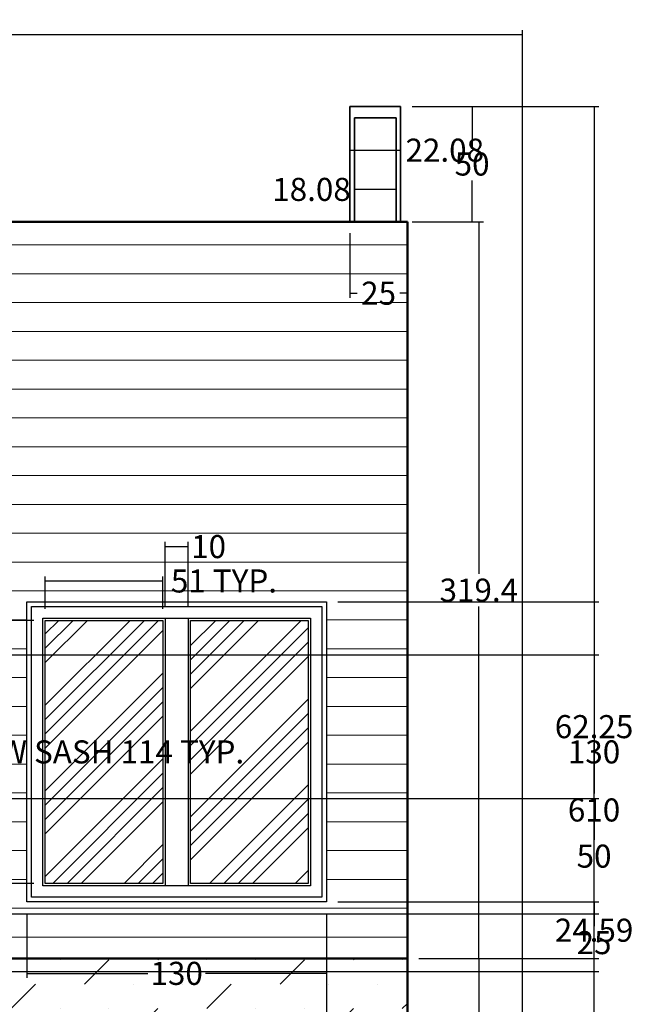
# Model space of a CAD drawing. Units: millimetres. Extents: x 301 to 1039, y -12 to 673.
# Tile 6 of 6: x 736 to 1002, y 246 to 673. Entities that reach past the tile are written whole.
import ezdxf

# ---------------------------------------------------------------- set-up
doc = ezdxf.new("R2010")
doc.units = ezdxf.units.MM
doc.header["$MEASUREMENT"] = 0
for name, color, linetype, lineweight in [('A-ANNO-DIMS', 2, 'Continuous', 18), ('A-GLAZ', 4, 'Continuous', 25), ('A-GLAZ-PATT', 8, 'Continuous', 13), ('A-ROOF', 1, 'Continuous', 35), ('A-WALL', 7, 'Continuous', 50), ('A-WALL-PATT', 9, 'Continuous', 13)]:
    doc.layers.add(name, color=color, linetype=linetype, lineweight=lineweight)
doc.styles.get("Standard").update_dxf_attribs({"font": 'arial.ttf'})
doc.dimstyles.get("Standard").update_dxf_attribs({"dimtxt": 10, "dimasz": 0.18, "dimexe": 2, "dimexo": 5, "dimgap": 2, "dimtad": 0, "dimtih": 1, "dimtoh": 1, "dimdec": 0, "dimzin": 0, "dimdsep": 46, "dimtxsty": 'Standard', "dimcen": 0.09, "dimadec": 0, "dimazin": 0, "dimtfac": 1, "dimtdec": 0, "dimtofl": 0, "dimtmove": 0, "dimatfit": 3, "dimfxl": 1, "dimtolj": 1, "dimtzin": 0, "dimarcsym": 0})

# ---------------------------------------------------------------- blocks, each defined once
blk = doc.blocks.new('WIN-SASH-SLIDING')
blk.add_line((51, 114), (51, 0))
blk.add_lwpolyline([(51, 0), (0, 0), (0, 114), (51, 114)])
blk = doc.blocks.new('*D16')
at = {"layer": 'A-ANNO-DIMS', "color": 0, "lineweight": -2, "transparency": 16777216}
for p, q in [((741.69, 412.26), (727.59, 412.26)), ((729.59, 412.08), (729.59, 362.44)), ((729.59, 298.44), (729.59, 348.09)), ((741.69, 298.26), (727.59, 298.26))]:
    blk.add_line(p, q, dxfattribs=at)
at = {"layer": 'A-ANNO-DIMS', "color": 0, "transparency": 16777216}
for points in [[(729.56, 412.08), (729.62, 412.08), (729.59, 412.26)], [(729.56, 298.44), (729.62, 298.44), (729.59, 298.26)]]:
    blk.add_solid(points, dxfattribs=at)
at = {"layer": 'Defpoints', "color": 0, "transparency": 16777216}
for p in [(729.59, 412.26), (746.69, 412.26), (746.69, 298.26)]:
    blk.add_point(p, dxfattribs=at)
at = {"layer": 'A-ANNO-DIMS', "color": 0, "transparency": 16777216, "insert": (729.59, 355.26), "char_height": 10, "attachment_point": 5}
blk.add_mtext('\\A1;SLIDING WINDOW SASH 114 TYP.', dxfattribs=at)
blk = doc.blocks.new('*D17')
at = {"layer": 'A-ANNO-DIMS', "color": 0, "lineweight": -2, "transparency": 16777216}
for p, q in [((746.69, 417.26), (746.69, 431.36)), ((797.69, 417.26), (797.69, 431.36)), ((746.87, 429.36), (797.51, 429.36)), ((797.69, 429.36), (797.87, 429.36))]:
    blk.add_line(p, q, dxfattribs=at)
at = {"layer": 'A-ANNO-DIMS', "color": 0, "transparency": 16777216}
for points in [[(746.87, 429.39), (746.87, 429.33), (746.69, 429.36)], [(797.51, 429.39), (797.51, 429.33), (797.69, 429.36)]]:
    blk.add_solid(points, dxfattribs=at)
at = {"layer": 'Defpoints', "color": 0, "transparency": 16777216}
for p in [(797.69, 429.36), (746.69, 412.26), (797.69, 412.26)]:
    blk.add_point(p, dxfattribs=at)
at = {"layer": 'A-ANNO-DIMS', "color": 0, "transparency": 16777216, "insert": (824.21, 429.36), "char_height": 10, "attachment_point": 5}
blk.add_mtext('\\A1;51 TYP.', dxfattribs=at)
blk = doc.blocks.new('*D20')
at = {"layer": 'A-ANNO-DIMS', "color": 0, "lineweight": -2, "transparency": 16777216}
for p, q in [((343.79, 30.09), (343.79, 668.09)), ((343.97, 666.09), (635.73, 666.09)), ((953.61, 666.09), (661.85, 666.09)), ((953.79, 30.09), (953.79, 668.09))]:
    blk.add_line(p, q, dxfattribs=at)
at = {"layer": 'A-ANNO-DIMS', "color": 0, "transparency": 16777216}
for points in [[(343.97, 666.12), (343.97, 666.06), (343.79, 666.09)], [(953.61, 666.12), (953.61, 666.06), (953.79, 666.09)]]:
    blk.add_solid(points, dxfattribs=at)
at = {"layer": 'Defpoints', "color": 0, "transparency": 16777216}
for p in [(953.79, 666.09), (343.79, 25.09), (953.79, 25.09)]:
    blk.add_point(p, dxfattribs=at)
at = {"layer": 'A-ANNO-DIMS', "color": 0, "transparency": 16777216, "insert": (648.79, 666.09), "char_height": 10, "attachment_point": 5}
blk.add_mtext('\\A1;610', dxfattribs=at)
blk = doc.blocks.new('*D21')
at = {"layer": 'A-ANNO-DIMS', "color": 0, "lineweight": -2, "transparency": 16777216}
for p, q in [((905.87, 635.09), (986.79, 635.09)), ((984.79, 634.91), (984.79, 337.19)), ((984.79, 25.27), (984.79, 322.98)), ((958.79, 25.09), (986.79, 25.09))]:
    blk.add_line(p, q, dxfattribs=at)
at = {"layer": 'A-ANNO-DIMS', "color": 0, "transparency": 16777216}
for points in [[(984.76, 634.91), (984.82, 634.91), (984.79, 635.09)], [(984.76, 25.27), (984.82, 25.27), (984.79, 25.09)]]:
    blk.add_solid(points, dxfattribs=at)
at = {"layer": 'Defpoints', "color": 0, "transparency": 16777216}
for p in [(900.87, 635.09), (984.79, 635.09), (953.79, 25.09)]:
    blk.add_point(p, dxfattribs=at)
at = {"layer": 'A-ANNO-DIMS', "color": 0, "transparency": 16777216, "insert": (984.79, 330.09), "char_height": 10, "attachment_point": 5}
blk.add_mtext('\\A1;610', dxfattribs=at)
blk = doc.blocks.new('*D38')
at = {"layer": 'A-ANNO-DIMS', "color": 0, "lineweight": -2, "transparency": 16777216}
for p, q in [((908.79, 265.67), (936.79, 265.67)), ((934.79, 265.49), (934.79, 157.49)), ((934.79, 35.27), (934.79, 143.27)), ((908.79, 35.09), (936.79, 35.09))]:
    blk.add_line(p, q, dxfattribs=at)
at = {"layer": 'A-ANNO-DIMS', "color": 0, "transparency": 16777216}
for points in [[(934.76, 265.49), (934.82, 265.49), (934.79, 265.67)], [(934.76, 35.27), (934.82, 35.27), (934.79, 35.09)]]:
    blk.add_solid(points, dxfattribs=at)
at = {"layer": 'Defpoints', "color": 0, "transparency": 16777216}
for p in [(903.79, 265.67), (903.79, 35.09), (934.79, 35.09)]:
    blk.add_point(p, dxfattribs=at)
at = {"layer": 'A-ANNO-DIMS', "color": 0, "transparency": 16777216, "insert": (934.79, 150.38), "char_height": 10, "attachment_point": 5}
blk.add_mtext('\\A1;230.6', dxfattribs=at)
blk = doc.blocks.new('*D39')
at = {"layer": 'A-ANNO-DIMS', "color": 0, "lineweight": -2, "transparency": 16777216}
for p, q in [((908.79, 585.09), (936.79, 585.09)), ((934.79, 584.91), (934.79, 432.49)), ((934.79, 265.85), (934.79, 418.27)), ((908.79, 265.67), (936.79, 265.67))]:
    blk.add_line(p, q, dxfattribs=at)
at = {"layer": 'A-ANNO-DIMS', "color": 0, "transparency": 16777216}
for points in [[(934.76, 584.91), (934.82, 584.91), (934.79, 585.09)], [(934.76, 265.85), (934.82, 265.85), (934.79, 265.67)]]:
    blk.add_solid(points, dxfattribs=at)
at = {"layer": 'Defpoints', "color": 0, "transparency": 16777216}
for p in [(903.79, 585.09), (903.79, 265.67), (934.79, 265.67)]:
    blk.add_point(p, dxfattribs=at)
at = {"layer": 'A-ANNO-DIMS', "color": 0, "transparency": 16777216, "insert": (934.79, 425.38), "char_height": 10, "attachment_point": 5}
blk.add_mtext('\\A1;319.4', dxfattribs=at)
blk = doc.blocks.new('*D46')
at = {"layer": 'A-ANNO-DIMS', "color": 0, "lineweight": -2, "transparency": 16777216}
for p, q in [((878.79, 590.09), (878.79, 618.09)), ((878.97, 616.09), (900.69, 616.09)), ((900.87, 590.09), (900.87, 618.09)), ((900.87, 616.09), (901.05, 616.09))]:
    blk.add_line(p, q, dxfattribs=at)
at = {"layer": 'A-ANNO-DIMS', "color": 0, "transparency": 16777216}
for points in [[(878.97, 616.12), (878.97, 616.06), (878.79, 616.09)], [(900.69, 616.12), (900.69, 616.06), (900.87, 616.09)]]:
    blk.add_solid(points, dxfattribs=at)
at = {"layer": 'Defpoints', "color": 0, "transparency": 16777216}
for p in [(900.87, 616.09), (878.79, 585.09), (900.87, 585.09)]:
    blk.add_point(p, dxfattribs=at)
at = {"layer": 'A-ANNO-DIMS', "color": 0, "transparency": 16777216, "insert": (920.02, 616.09), "char_height": 10, "attachment_point": 5}
blk.add_mtext('\\A1;22.08', dxfattribs=at)
blk = doc.blocks.new('*D47')
at = {"layer": 'A-ANNO-DIMS', "color": 0, "lineweight": -2, "transparency": 16777216}
for p, q in [((880.79, 625.09), (880.79, 597.09)), ((898.87, 625.09), (898.87, 597.09)), ((880.79, 599.09), (880.61, 599.09)), ((898.69, 599.09), (880.97, 599.09))]:
    blk.add_line(p, q, dxfattribs=at)
at = {"layer": 'A-ANNO-DIMS', "color": 0, "transparency": 16777216}
for points in [[(880.97, 599.12), (880.97, 599.06), (880.79, 599.09)], [(898.69, 599.12), (898.69, 599.06), (898.87, 599.09)]]:
    blk.add_solid(points, dxfattribs=at)
at = {"layer": 'Defpoints', "color": 0, "transparency": 16777216}
for p in [(880.79, 630.09), (898.87, 630.09), (880.79, 599.09)]:
    blk.add_point(p, dxfattribs=at)
at = {"layer": 'A-ANNO-DIMS', "color": 0, "transparency": 16777216, "insert": (862.2, 599.09), "char_height": 10, "attachment_point": 5}
blk.add_mtext('\\A1;18.08', dxfattribs=at)
blk = doc.blocks.new('*D48')
at = {"layer": 'A-ANNO-DIMS', "color": 0, "lineweight": -2, "transparency": 16777216}
for p, q in [((878.79, 580.09), (878.79, 552.09)), ((903.79, 580.09), (903.79, 552.09)), ((878.97, 554.09), (882, 554.09)), ((903.61, 554.09), (900.57, 554.09))]:
    blk.add_line(p, q, dxfattribs=at)
at = {"layer": 'A-ANNO-DIMS', "color": 0, "transparency": 16777216}
for points in [[(878.97, 554.12), (878.97, 554.06), (878.79, 554.09)], [(903.61, 554.12), (903.61, 554.06), (903.79, 554.09)]]:
    blk.add_solid(points, dxfattribs=at)
at = {"layer": 'Defpoints', "color": 0, "transparency": 16777216}
for p in [(878.79, 585.09), (903.79, 585.09), (878.79, 554.09)]:
    blk.add_point(p, dxfattribs=at)
at = {"layer": 'A-ANNO-DIMS', "color": 0, "transparency": 16777216, "insert": (891.29, 554.09), "char_height": 10, "attachment_point": 5}
blk.add_mtext('\\A1;25', dxfattribs=at)
blk = doc.blocks.new('*D49')
at = {"layer": 'A-ANNO-DIMS', "color": 0, "lineweight": -2, "transparency": 16777216}
for p, q in [((905.87, 635.09), (933.87, 635.09)), ((931.87, 634.91), (931.87, 617.19)), ((931.87, 585.27), (931.87, 602.98)), ((905.87, 585.09), (933.87, 585.09))]:
    blk.add_line(p, q, dxfattribs=at)
at = {"layer": 'A-ANNO-DIMS', "color": 0, "transparency": 16777216}
for points in [[(931.84, 634.91), (931.9, 634.91), (931.87, 635.09)], [(931.84, 585.27), (931.9, 585.27), (931.87, 585.09)]]:
    blk.add_solid(points, dxfattribs=at)
at = {"layer": 'Defpoints', "color": 0, "transparency": 16777216}
for p in [(900.87, 635.09), (900.87, 585.09), (931.87, 585.09)]:
    blk.add_point(p, dxfattribs=at)
at = {"layer": 'A-ANNO-DIMS', "color": 0, "transparency": 16777216, "insert": (931.87, 610.09), "char_height": 10, "attachment_point": 5}
blk.add_mtext('\\A1;50', dxfattribs=at)
blk = doc.blocks.new('*D55')
at = {"layer": 'A-ANNO-DIMS', "color": 0, "lineweight": -2, "transparency": 16777216}
for p, q in [((718.79, 285.09), (986.79, 285.09)), ((984.79, 284.91), (984.79, 279.69)), ((984.79, 260.27), (984.79, 265.48)), ((718.79, 260.09), (986.79, 260.09))]:
    blk.add_line(p, q, dxfattribs=at)
at = {"layer": 'A-ANNO-DIMS', "color": 0, "transparency": 16777216}
for points in [[(984.76, 284.91), (984.82, 284.91), (984.79, 285.09)], [(984.76, 260.27), (984.82, 260.27), (984.79, 260.09)]]:
    blk.add_solid(points, dxfattribs=at)
at = {"layer": 'Defpoints', "color": 0, "transparency": 16777216}
for p in [(713.79, 285.09), (984.79, 285.09), (713.79, 260.09)]:
    blk.add_point(p, dxfattribs=at)
at = {"layer": 'A-ANNO-DIMS', "color": 0, "transparency": 16777216, "insert": (984.79, 272.59), "char_height": 10, "attachment_point": 5}
blk.add_mtext('\\A1;25', dxfattribs=at)
blk = doc.blocks.new('*D56')
at = {"layer": 'A-ANNO-DIMS', "color": 0, "lineweight": -2, "transparency": 16777216}
for p, q in [((718.79, 335.09), (986.79, 335.09)), ((984.79, 334.91), (984.79, 317.19)), ((984.79, 285.27), (984.79, 302.98)), ((718.79, 285.09), (986.79, 285.09))]:
    blk.add_line(p, q, dxfattribs=at)
at = {"layer": 'A-ANNO-DIMS', "color": 0, "transparency": 16777216}
for points in [[(984.76, 334.91), (984.82, 334.91), (984.79, 335.09)], [(984.76, 285.27), (984.82, 285.27), (984.79, 285.09)]]:
    blk.add_solid(points, dxfattribs=at)
at = {"layer": 'Defpoints', "color": 0, "transparency": 16777216}
for p in [(713.79, 335.09), (984.79, 335.09), (713.79, 285.09)]:
    blk.add_point(p, dxfattribs=at)
at = {"layer": 'A-ANNO-DIMS', "color": 0, "transparency": 16777216, "insert": (984.79, 310.09), "char_height": 10, "attachment_point": 5}
blk.add_mtext('\\A1;50', dxfattribs=at)
blk = doc.blocks.new('*D57')
at = {"layer": 'A-ANNO-DIMS', "color": 0, "lineweight": -2, "transparency": 16777216}
for p, q in [((671.29, 397.33), (986.79, 397.33)), ((984.79, 397.15), (984.79, 373.32)), ((984.79, 335.27), (984.79, 359.11)), ((718.79, 335.09), (986.79, 335.09))]:
    blk.add_line(p, q, dxfattribs=at)
at = {"layer": 'A-ANNO-DIMS', "color": 0, "transparency": 16777216}
for points in [[(984.76, 397.15), (984.82, 397.15), (984.79, 397.33)], [(984.76, 335.27), (984.82, 335.27), (984.79, 335.09)]]:
    blk.add_solid(points, dxfattribs=at)
at = {"layer": 'Defpoints', "color": 0, "transparency": 16777216}
for p in [(666.29, 397.33), (984.79, 397.33), (713.79, 335.09)]:
    blk.add_point(p, dxfattribs=at)
at = {"layer": 'A-ANNO-DIMS', "color": 0, "transparency": 16777216, "insert": (984.79, 366.21), "char_height": 10, "attachment_point": 5}
blk.add_mtext('\\A1;62.25', dxfattribs=at)
blk = doc.blocks.new('*D74')
at = {"layer": 'A-ANNO-DIMS', "color": 0, "lineweight": -2, "transparency": 16777216}
for p, q in [((738.69, 285.26), (738.69, 257.26)), ((868.69, 285.26), (868.69, 257.26)), ((738.87, 259.26), (791.13, 259.26)), ((868.51, 259.26), (816.25, 259.26))]:
    blk.add_line(p, q, dxfattribs=at)
at = {"layer": 'A-ANNO-DIMS', "color": 0, "transparency": 16777216}
for points in [[(738.87, 259.29), (738.87, 259.23), (738.69, 259.26)], [(868.51, 259.29), (868.51, 259.23), (868.69, 259.26)]]:
    blk.add_solid(points, dxfattribs=at)
at = {"layer": 'Defpoints', "color": 0, "transparency": 16777216}
for p in [(738.69, 290.26), (868.69, 290.26), (738.69, 259.26)]:
    blk.add_point(p, dxfattribs=at)
at = {"layer": 'A-ANNO-DIMS', "color": 0, "transparency": 16777216, "insert": (803.69, 259.26), "char_height": 10, "attachment_point": 5}
blk.add_mtext('\\A1;130', dxfattribs=at)
blk = doc.blocks.new('*D75')
at = {"layer": 'A-ANNO-DIMS', "color": 0, "lineweight": -2, "transparency": 16777216}
for p, q in [((868.69, 285.26), (868.69, -7.91)), ((903.79, 260.67), (903.79, -7.91)), ((868.87, -5.91), (872.22, -5.91)), ((903.61, -5.91), (900.26, -5.91))]:
    blk.add_line(p, q, dxfattribs=at)
at = {"layer": 'A-ANNO-DIMS', "color": 0, "transparency": 16777216}
for points in [[(868.87, -5.88), (868.87, -5.94), (868.69, -5.91)], [(903.61, -5.88), (903.61, -5.94), (903.79, -5.91)]]:
    blk.add_solid(points, dxfattribs=at)
at = {"layer": 'Defpoints', "color": 0, "transparency": 16777216}
for p in [(868.69, 290.26), (903.79, 265.67), (903.79, -5.91)]:
    blk.add_point(p, dxfattribs=at)
at = {"layer": 'A-ANNO-DIMS', "color": 0, "transparency": 16777216, "insert": (886.24, -5.91), "char_height": 10, "attachment_point": 5}
blk.add_mtext('\\A1;35.1', dxfattribs=at)
blk = doc.blocks.new('*D76')
at = {"layer": 'A-ANNO-DIMS', "color": 0, "lineweight": -2, "transparency": 16777216}
for p, q in [((873.69, 290.26), (986.79, 290.26)), ((984.79, 290.08), (984.79, 285.07)), ((984.79, 265.85), (984.79, 270.86)), ((908.79, 265.67), (986.79, 265.67))]:
    blk.add_line(p, q, dxfattribs=at)
at = {"layer": 'A-ANNO-DIMS', "color": 0, "transparency": 16777216}
for points in [[(984.76, 290.08), (984.82, 290.08), (984.79, 290.26)], [(984.76, 265.85), (984.82, 265.85), (984.79, 265.67)]]:
    blk.add_solid(points, dxfattribs=at)
at = {"layer": 'Defpoints', "color": 0, "transparency": 16777216}
for p in [(868.69, 290.26), (984.79, 290.26), (903.79, 265.67)]:
    blk.add_point(p, dxfattribs=at)
at = {"layer": 'A-ANNO-DIMS', "color": 0, "transparency": 16777216, "insert": (984.79, 277.97), "char_height": 10, "attachment_point": 5}
blk.add_mtext('\\A1;24.59', dxfattribs=at)
blk = doc.blocks.new('*D77')
at = {"layer": 'A-ANNO-DIMS', "color": 0, "lineweight": -2, "transparency": 16777216}
for p, q in [((873.69, 420.26), (986.79, 420.26)), ((984.79, 420.08), (984.79, 362.37)), ((984.79, 290.44), (984.79, 348.15)), ((873.69, 290.26), (986.79, 290.26))]:
    blk.add_line(p, q, dxfattribs=at)
at = {"layer": 'A-ANNO-DIMS', "color": 0, "transparency": 16777216}
for points in [[(984.76, 420.08), (984.82, 420.08), (984.79, 420.26)], [(984.76, 290.44), (984.82, 290.44), (984.79, 290.26)]]:
    blk.add_solid(points, dxfattribs=at)
at = {"layer": 'Defpoints', "color": 0, "transparency": 16777216}
for p in [(868.69, 420.26), (984.79, 420.26), (868.69, 290.26)]:
    blk.add_point(p, dxfattribs=at)
at = {"layer": 'A-ANNO-DIMS', "color": 0, "transparency": 16777216, "insert": (984.79, 355.26), "char_height": 10, "attachment_point": 5}
blk.add_mtext('\\A1;130', dxfattribs=at)
blk = doc.blocks.new('*D78')
at = {"layer": 'A-ANNO-DIMS', "color": 0, "lineweight": -2, "transparency": 16777216}
for p, q in [((798.69, 418.26), (798.69, 446.26)), ((798.87, 444.26), (808.51, 444.26)), ((808.69, 418.26), (808.69, 446.26)), ((808.69, 444.26), (808.87, 444.26))]:
    blk.add_line(p, q, dxfattribs=at)
at = {"layer": 'A-ANNO-DIMS', "color": 0, "transparency": 16777216}
for points in [[(798.87, 444.29), (798.87, 444.23), (798.69, 444.26)], [(808.51, 444.29), (808.51, 444.23), (808.69, 444.26)]]:
    blk.add_solid(points, dxfattribs=at)
at = {"layer": 'Defpoints', "color": 0, "transparency": 16777216}
for p in [(808.69, 444.26), (798.69, 413.26), (808.69, 413.26)]:
    blk.add_point(p, dxfattribs=at)
at = {"layer": 'A-ANNO-DIMS', "color": 0, "transparency": 16777216, "insert": (817.54, 444.26), "char_height": 10, "attachment_point": 5}
blk.add_mtext('\\A1;10', dxfattribs=at)

msp = doc.modelspace()

# ---------------------------------------------------------------- hatches: boundary and pattern name
at = {"layer": 'A-GLAZ-PATT'}
h = msp.add_hatch(dxfattribs=at)
h.set_pattern_fill('ANSI34', color=256, scale=35)
h.paths.add_polyline_path([(528.788, 400.52), (528.788, 425.088), (463.788, 425.088), (463.788, 400.52), (463.788, 335.088), (528.788, 335.088)])
h.paths.add_polyline_path([(494.288, 333.088), (463.788, 333.088), (463.788, 300.088), (494.288, 300.088)])
h.paths.add_polyline_path([(528.788, 333.088), (496.288, 333.088), (496.288, 300.088), (528.788, 300.088)])
h.paths.add_polyline_path([(618.788, 400.52), (618.788, 425.088), (553.788, 425.088), (553.788, 400.52), (553.788, 335.088), (618.788, 335.088)])
h.paths.add_polyline_path([(618.788, 333.088), (574.798, 333.088), (574.798, 300.088), (618.788, 300.088)])
h.paths.add_polyline_path([(572.798, 333.088), (553.788, 333.088), (553.788, 300.088), (572.798, 300.088)])
h.paths.add_polyline_path([(501.288, 180.088), (433.788, 180.088), (433.788, 110.088), (501.288, 110.088)])
h.paths.add_polyline_path([(573.788, 180.088), (506.288, 180.088), (506.288, 110.088), (573.788, 110.088)])
h.paths.add_polyline_path([(573.788, 210.088), (506.288, 210.088), (506.288, 185.088), (573.788, 185.088)])
h.paths.add_polyline_path([(501.288, 210.088), (433.788, 210.088), (433.788, 185.088), (501.288, 185.088)])
h.paths.add_polyline_path([(797.687, 412.264), (746.687, 412.264), (746.687, 298.264), (797.687, 298.264)])
h.paths.add_polyline_path([(860.687, 412.264), (809.687, 412.264), (809.687, 298.264), (860.687, 298.264)])
at = {"layer": 'A-WALL-PATT'}
h = msp.add_hatch(dxfattribs=at)
h.set_pattern_fill('ANSI31', color=256, scale=100, angle=135)
h.paths.add_polyline_path([(903.788, 585.088), (703.788, 585.088), (703.788, 535.088), (723.788, 535.088), (723.788, 505.088), (703.788, 505.088), (703.788, 335.088), (713.788, 335.088), (713.788, 333.088), (703.788, 333.088), (703.788, 285.088), (713.788, 285.088), (713.788, 265.672), (903.788, 265.672)])
h.paths.add_polyline_path([(868.687, 420.264), (868.687, 290.264), (738.687, 290.264), (738.687, 420.264)], flags=16)
h.paths.add_polyline_path([(866.687, 418.264), (866.687, 292.264), (740.687, 292.264), (740.687, 418.264)], flags=0)
h.paths.add_polyline_path([(861.687, 413.264), (861.687, 297.264), (745.687, 297.264), (745.687, 413.264)], flags=0)
h.paths.add_polyline_path([(860.687, 412.264), (860.687, 298.264), (809.687, 298.264), (809.687, 412.264)], flags=0)
h.paths.add_polyline_path([(797.687, 412.264), (797.687, 298.264), (746.687, 298.264), (746.687, 412.264)], flags=0)
h = msp.add_hatch(dxfattribs=at)
h.set_pattern_fill('MUDST', color=256, scale=60, angle=45)
edge = h.paths.add_edge_path()
edge.add_line((703.788, 505.088), (403.788, 505.088))
edge.add_line((403.788, 505.088), (403.788, 335.088))
edge.add_line((403.788, 335.088), (448.788, 335.088))
edge.add_line((448.788, 335.088), (448.788, 400.52))
edge.add_line((448.788, 400.52), (448.788, 440.088))
edge.add_line((448.788, 440.088), (633.788, 440.088))
edge.add_line((633.788, 440.088), (633.788, 400.52))
edge.add_line((633.788, 400.52), (633.788, 335.088))
edge.add_line((633.788, 335.088), (673.88, 335.088))
edge.add_spline(control_points=[(673.88, 335.088), (673.929, 335.734), (674.283, 339.462), (675.587, 346.794), (678.602, 339.909), (679.226, 336.718), (679.369, 335.088)], knot_values=[26.7052686, 26.7052686, 26.7052686, 26.7052686, 28.3156814, 35.5227919, 39.6456178, 44.5318346, 44.5318346, 44.5318346, 44.5318346], degree=3, periodic=0)
edge.add_line((679.369, 335.088), (703.788, 335.088))
edge.add_line((703.788, 335.088), (703.788, 505.088))
h.paths.add_polyline_path([(681.292, 397.334, -1), (651.292, 397.334, -1)], flags=16)
h.paths.add_polyline_path([(679.292, 397.334, -1), (653.292, 397.334, -1)], flags=0)
h.paths.add_polyline_path([(448.788, 333.088), (403.788, 333.088), (403.788, 285.088), (448.788, 285.088)])
h.paths.add_polyline_path([(613.788, 260.088), (713.788, 260.088), (713.788, 285.088), (403.788, 285.088), (393.788, 285.088), (393.788, 35.088), (403.788, 35.088), (613.788, 35.088)])
h.paths.add_polyline_path([(578.788, 215.088), (578.788, 105.088), (428.788, 105.088), (428.788, 215.088)], flags=16)
h.paths.add_polyline_path([(501.288, 210.088), (501.288, 185.088), (433.788, 185.088), (433.788, 210.088)], flags=0)
h.paths.add_polyline_path([(501.288, 180.088), (501.288, 110.088), (433.788, 110.088), (433.788, 180.088)], flags=0)
h.paths.add_polyline_path([(506.288, 210.088), (573.788, 210.088), (573.788, 185.088), (506.288, 185.088)], flags=0)
h.paths.add_polyline_path([(506.288, 180.088), (573.788, 180.088), (573.788, 110.088), (506.288, 110.088)], flags=0)
edge = h.paths.add_edge_path()
edge.add_spline(control_points=[(675.148, 309.006), (675.282, 309.92), (671.965, 311.304), (670.019, 313.17), (668.379, 316.485), (667.076, 320.028), (669.149, 324.142), (672.687, 322.877), (673.644, 321.553), (673.786, 321.296)], knot_values=[12.4980994, 12.4980994, 12.4980994, 12.4980994, 15.7345293, 18.1242776, 22.0598536, 26.1694355, 29.2709867, 33.3603853, 34.273637, 34.273637, 34.273637, 34.273637], degree=3, periodic=0)
edge.add_spline(control_points=[(673.786, 321.296), (673.373, 322.666), (672.565, 324.662), (673.805, 325.84), (674.246, 326.099)], knot_values=[12.3304253, 12.3304253, 12.3304253, 12.3304253, 16.1943692, 17.6683934, 17.6683934, 17.6683934, 17.6683934], degree=3, periodic=0)
edge.add_spline(control_points=[(674.246, 326.099), (673.92, 328.298), (673.697, 330.39), (673.774, 333.088)], knot_values=[46.2924512, 46.2924512, 46.2924512, 46.2924512, 53.8278009, 53.8278009, 53.8278009, 53.8278009], degree=3, periodic=0)
edge.add_line((673.774, 333.088), (648.788, 333.088))
edge.add_line((648.788, 333.088), (648.788, 285.088))
edge.add_line((648.788, 285.088), (666.788, 285.088))
edge.add_line((666.788, 285.088), (664.215, 309.96))
edge.add_arc((676.288, 385.148), 76.15, 260.87778, 269.14183)
edge = h.paths.add_edge_path()
edge.add_line((703.788, 333.088), (679.453, 333.088))
edge.add_spline(control_points=[(679.453, 333.088), (679.452, 331.277), (679.21, 329.205), (678.936, 327.067), (678.889, 326.706)], knot_values=[17.8386285, 17.8386285, 17.8386285, 17.8386285, 23.5111371, 24.6594022, 24.6594022, 24.6594022, 24.6594022], degree=3, periodic=0)
edge.add_spline(control_points=[(678.889, 326.706), (678.729, 326.741), (678.565, 326.771), (678.396, 326.794)], knot_values=[21.2892091, 21.2892091, 21.2892091, 21.2892091, 21.7264211, 21.7264211, 21.7264211, 21.7264211], degree=3, periodic=0)
edge.add_spline(control_points=[(678.396, 326.794), (678.233, 326.816), (678.067, 326.832), (677.898, 326.842)], knot_values=[20.8675669, 20.8675669, 20.8675669, 20.8675669, 21.2892091, 21.2892091, 21.2892091, 21.2892091], degree=3, periodic=0)
edge.add_spline(control_points=[(677.898, 326.842), (676.995, 326.898), (676.024, 326.786), (675.195, 326.517)], knot_values=[18.611077, 18.611077, 18.611077, 18.611077, 20.8675669, 20.8675669, 20.8675669, 20.8675669], degree=3, periodic=0)
edge.add_spline(control_points=[(675.195, 326.517), (675.029, 326.464), (674.869, 326.404), (674.716, 326.337)], knot_values=[18.1593829, 18.1593829, 18.1593829, 18.1593829, 18.611077, 18.611077, 18.611077, 18.611077], degree=3, periodic=0)
edge.add_spline(control_points=[(674.716, 326.337), (674.55, 326.265), (674.392, 326.186), (674.246, 326.099)], knot_values=[17.6683934, 17.6683934, 17.6683934, 17.6683934, 18.1593829, 18.1593829, 18.1593829, 18.1593829], degree=3, periodic=0)
edge.add_spline(control_points=[(674.246, 326.099), (673.805, 325.84), (672.565, 324.662), (673.373, 322.666), (673.786, 321.296)], knot_values=[12.3304253, 12.3304253, 12.3304253, 12.3304253, 13.8044495, 17.6683934, 17.6683934, 17.6683934, 17.6683934], degree=3, periodic=0)
edge.add_spline(control_points=[(673.786, 321.296), (674.162, 320.613), (674.301, 319.823), (674.341, 318.987)], knot_values=[10.0649388, 10.0649388, 10.0649388, 10.0649388, 12.4980994, 12.4980994, 12.4980994, 12.4980994], degree=3, periodic=0)
edge.add_spline(control_points=[(674.341, 318.987), (674.206, 319.737), (674.024, 320.504), (673.786, 321.296)], knot_values=[10.094462, 10.094462, 10.094462, 10.094462, 12.3304253, 12.3304253, 12.3304253, 12.3304253], degree=3, periodic=0)
edge.add_spline(control_points=[(673.786, 321.296), (673.644, 321.553), (672.687, 322.877), (669.149, 324.142), (667.076, 320.028), (668.379, 316.485), (670.019, 313.17), (671.965, 311.304), (675.282, 309.92), (675.148, 309.006)], knot_values=[12.4980994, 12.4980994, 12.4980994, 12.4980994, 13.4113511, 17.5007497, 20.6023009, 24.7118828, 28.6474588, 31.0372071, 34.273637, 34.273637, 34.273637, 34.273637], degree=3, periodic=0)
edge.add_arc((676.288, 385.148), 76.15, 260.87778, 269.14183, ccw=False)
edge.add_line((664.215, 309.96), (666.788, 285.088))
edge.add_line((666.788, 285.088), (703.788, 285.088))
edge.add_line((703.788, 285.088), (703.788, 333.088))
h.paths.add_polyline_path([(687.234, 308.777), (684.887, 286.088), (667.69, 286.088), (665.343, 308.777, 0.0712952)], flags=16)
h.paths.add_polyline_path([(903.788, 265.672), (713.788, 265.672), (713.788, 260.088), (703.788, 260.088), (703.788, 35.088), (728.788, 35.088), (728.788, 160.088), (878.788, 160.088), (878.788, 35.088), (903.788, 35.088)])

# ---------------------------------------------------------------- linework, layer by layer
at = {"layer": 'A-GLAZ'}
for p, q in [((798.687, 413.264), (798.687, 297.264)), ((808.687, 413.264), (808.687, 297.264))]:
    msp.add_line(p, q, dxfattribs=at)
for points in [[(738.687, 420.264), (868.687, 420.264), (868.687, 290.264), (738.687, 290.264)], [(740.687, 418.264), (866.687, 418.264), (866.687, 292.264), (740.687, 292.264)], [(745.687, 413.264), (861.687, 413.264), (861.687, 297.264), (745.687, 297.264)]]:
    msp.add_lwpolyline(points, close=True, dxfattribs=at)
at = {"layer": 'A-ROOF'}
for p, q in [((900.87, 635.088), (878.788, 635.088)), ((878.788, 585.088), (878.788, 635.088)), ((900.87, 635.088), (900.87, 585.088)), ((880.788, 585.088), (880.788, 630.088)), ((898.87, 630.088), (880.788, 630.088)), ((898.87, 630.088), (898.87, 585.088))]:
    msp.add_line(p, q, dxfattribs=at)
at = {"layer": 'A-WALL'}
for p, q in [((903.788, 585.088), (703.788, 585.088)), ((903.788, 35.088), (903.788, 585.088)), ((713.788, 265.672), (903.788, 265.672))]:
    msp.add_line(p, q, dxfattribs=at)

# ---------------------------------------------------------------- block references
at = {"layer": 'A-GLAZ'}
msp.add_blockref('WIN-SASH-SLIDING', (746.687, 298.264), dxfattribs=at)
at = {"layer": 'A-GLAZ', "rotation": 180}
msp.add_blockref('WIN-SASH-SLIDING', (860.687, 412.264), dxfattribs=at)

# ---------------------------------------------------------------- dimensions: what is measured, and where the dimension line sits
at = {"layer": 'A-ANNO-DIMS'}
for base, p1, p2, override, picture, middle in [((953.788, 666.088), (343.788, 25.088), (953.788, 25.088), {"dimdec": 0, "dimlfac": 1, "dimrnd": 0, "dimzin": 0, "dimdsep": 46, "dimlunit": 2}, '*D20', (648.788, 666.088)), ((900.87, 616.088), (878.788, 585.088), (900.87, 585.088), {"dimdec": 2, "dimlfac": 1, "dimrnd": 0, "dimzin": 0, "dimdsep": 46, "dimlunit": 2}, '*D46', (920.018, 616.088)), ((808.687, 444.264), (798.687, 413.264), (808.687, 413.264), {"dimdec": 0, "dimlfac": 1, "dimrnd": 0, "dimzin": 0, "dimdsep": 46, "dimlunit": 2}, '*D78', (817.541, 444.264)), ((903.788, -5.912), (868.687, 290.264), (903.788, 265.672), {"dimdec": 1, "dimlfac": 1, "dimrnd": 0, "dimzin": 0, "dimdsep": 46, "dimlunit": 2}, '*D75', (886.238, -5.912))]:
    dim = msp.add_linear_dim(base=base, p1=p1, p2=p2, dimstyle='Standard', override=override, dxfattribs=at)
    dim.commit()
    dim.dimension.update_dxf_attribs({"geometry": picture, "text_midpoint": middle})
for base, p1, p2, angle, override, picture, middle in [((984.788, 635.088), (953.788, 25.088), (900.87, 635.088), 90, {"dimdec": 0, "dimlfac": 1, "dimrnd": 0, "dimzin": 0, "dimdsep": 46, "dimlunit": 2}, '*D21', (984.788, 330.088)), ((931.87, 585.088), (900.87, 635.088), (900.87, 585.088), 270, {"dimdec": 0, "dimlfac": 1, "dimrnd": 0, "dimzin": 0, "dimdsep": 46, "dimlunit": 2}, '*D49', (931.87, 610.088)), ((880.788, 599.088), (898.87, 630.088), (880.788, 630.088), 180, {"dimdec": 2, "dimlfac": 1, "dimrnd": 0, "dimzin": 0, "dimdsep": 46, "dimlunit": 2}, '*D47', (862.196, 599.088)), ((878.788, 554.088), (903.788, 585.088), (878.788, 585.088), 180, {"dimdec": 0, "dimlfac": 1, "dimrnd": 0, "dimzin": 0, "dimdsep": 46, "dimlunit": 2}, '*D48', (891.288, 554.088)), ((934.788, 265.672), (903.788, 585.088), (903.788, 265.672), 270, {"dimdec": 1, "dimlfac": 1, "dimrnd": 0, "dimzin": 0, "dimdsep": 46, "dimlunit": 2}, '*D39', (934.788, 425.38)), ((984.788, 420.264), (868.687, 290.264), (868.687, 420.264), 90, {"dimdec": 0, "dimlfac": 1, "dimrnd": 0, "dimzin": 0, "dimdsep": 46, "dimlunit": 2}, '*D77', (984.788, 355.264)), ((984.788, 397.334), (713.788, 335.088), (666.292, 397.334), 90, {"dimdec": 2, "dimlfac": 1, "dimrnd": 0, "dimzin": 0, "dimdsep": 46, "dimlunit": 2}, '*D57', (984.788, 366.211)), ((984.788, 335.088), (713.788, 285.088), (713.788, 335.088), 90, {"dimdec": 0, "dimlfac": 1, "dimrnd": 0, "dimzin": 0, "dimdsep": 46, "dimlunit": 2}, '*D56', (984.788, 310.088)), ((738.687, 259.264), (868.687, 290.264), (738.687, 290.264), 180, {"dimdec": 0, "dimlfac": 1, "dimrnd": 0, "dimzin": 0, "dimdsep": 46, "dimlunit": 2}, '*D74', (803.687, 259.264)), ((984.788, 290.264), (903.788, 265.672), (868.687, 290.264), 90, {"dimdec": 2, "dimlfac": 1, "dimrnd": 0, "dimzin": 0, "dimdsep": 46, "dimlunit": 2}, '*D76', (984.788, 277.968)), ((984.788, 285.088), (713.788, 260.088), (713.788, 285.088), 90, {"dimdec": 0, "dimlfac": 1, "dimrnd": 0, "dimzin": 0, "dimdsep": 46, "dimlunit": 2}, '*D55', (984.788, 272.588)), ((934.788, 35.088), (903.788, 265.672), (903.788, 35.088), 270, {"dimdec": 1, "dimlfac": 1, "dimrnd": 0, "dimzin": 0, "dimdsep": 46, "dimlunit": 2}, '*D38', (934.788, 150.38))]:
    dim = msp.add_linear_dim(base=base, p1=p1, p2=p2, angle=angle, dimstyle='Standard', override=override, dxfattribs=at)
    dim.commit()
    dim.dimension.update_dxf_attribs({"geometry": picture, "text_midpoint": middle})
dim = msp.add_linear_dim(base=(797.687, 429.364), p1=(746.687, 412.264), p2=(797.687, 412.264), text='<> TYP.', dimstyle='Standard', override={"dimdec": 0, "dimrnd": 0, "dimzin": 0, "dimlunit": 2}, dxfattribs=at)
dim.commit()
dim.dimension.update_dxf_attribs({"geometry": '*D17', "text_midpoint": (824.205, 429.364)})
dim = msp.add_linear_dim(base=(729.587, 412.264), p1=(746.687, 298.264), p2=(746.687, 412.264), angle=90, text='SLIDING WINDOW SASH <> TYP.', dimstyle='Standard', override={"dimdec": 0, "dimrnd": 0, "dimzin": 0, "dimlunit": 2}, dxfattribs=at)
dim.commit()
dim.dimension.update_dxf_attribs({"geometry": '*D16', "text_midpoint": (729.587, 355.264)})

doc.saveas('drawing.dxf')
